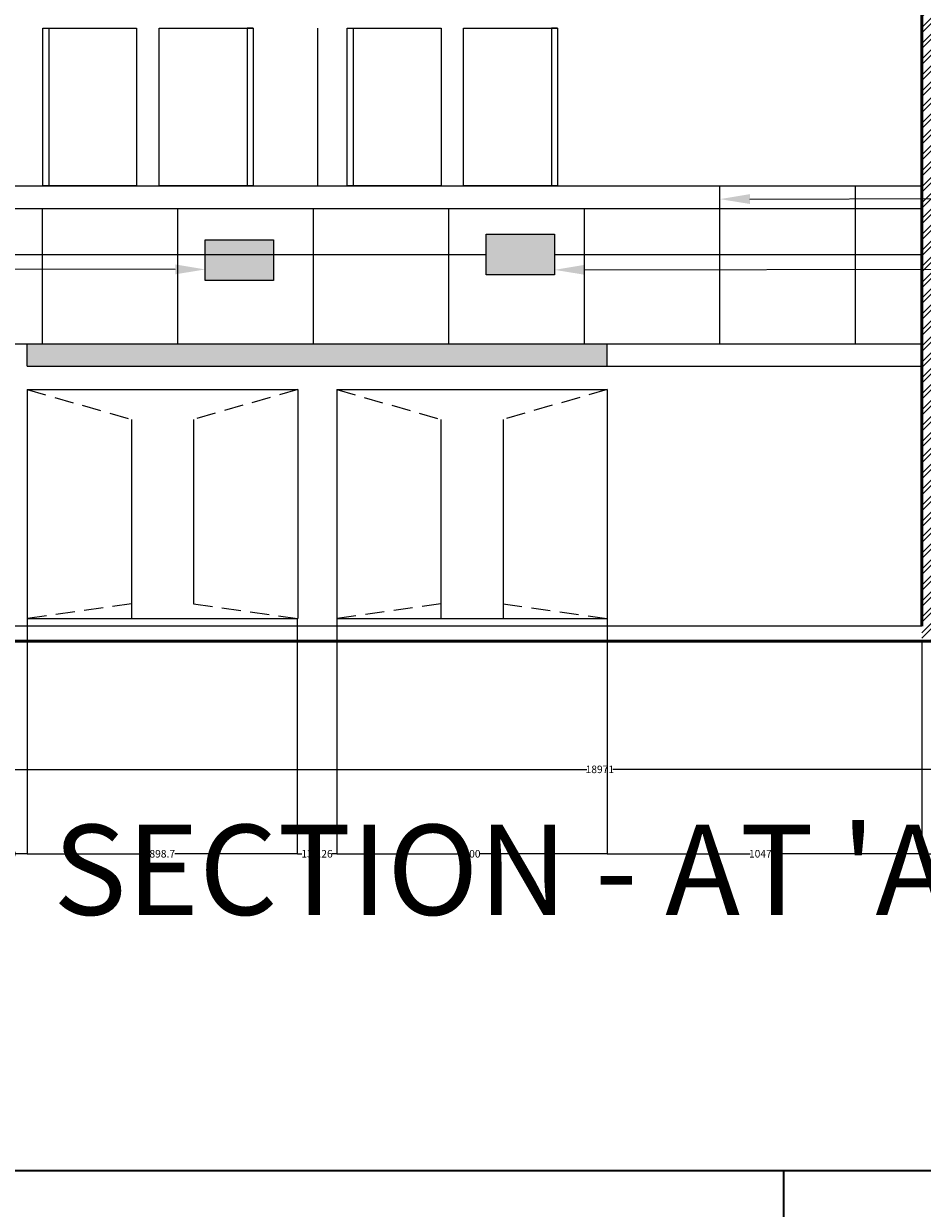
# Model space of a CAD drawing. Units: millimetres. Extents: x 1944 to 29915, y -10550 to 5909.
# Tile 15 of 24: x 13987 to 16977, y -1857 to 2086. Entities that reach past the tile are written whole.
import ezdxf
from ezdxf import colors
from ezdxf.entities.mleader import LeaderData, LeaderLine
from ezdxf.math import Vec2, Vec3

# ---------------------------------------------------------------- set-up
doc = ezdxf.new("R2010")
doc.units = ezdxf.units.MM
doc.header["$MEASUREMENT"] = 0
doc.linetypes.add('HIDDEN', pattern=[9.525, 6.35, -3.175])
for name, color, linetype, lineweight in [('A-ANNO-DIMS', 2, 'Continuous', 18), ('A-ANNO-TEXT', 7, 'Continuous', 25), ('A-ELEV', 3, 'Continuous', 18), ('A-ELEV-HIDN', 3, 'HIDDEN', 13), ('A-SECT', 7, 'Continuous', 35), ('A-WALL', 7, 'Continuous', 50), ('A-WALL-PATT', 8, 'Continuous', 18)]:
    doc.layers.add(name, color=color, linetype=linetype, lineweight=lineweight)
doc.styles.get("Standard").update_dxf_attribs({"font": 'arial.ttf'})
doc.dimstyles.get("Standard").update_dxf_attribs({"dimtxt": 25, "dimasz": 0.18, "dimexe": 0.18, "dimexo": 0.0625, "dimgap": 0.09, "dimtad": 0, "dimtih": 1, "dimtoh": 1, "dimdec": 0, "dimzin": 0, "dimdsep": 46, "dimtxsty": 'Standard', "dimcen": 0.09, "dimadec": 0, "dimazin": 0, "dimtfac": 1, "dimtdec": 0, "dimtofl": 0, "dimtmove": 0, "dimatfit": 3, "dimfxl": 1, "dimtolj": 1, "dimtzin": 0, "dimarcsym": 0})

# ---------------------------------------------------------------- blocks, each defined once
blk = doc.blocks.new('*D66')
at = {"layer": 'A-ANNO-DIMS', "color": 0, "lineweight": -2, "transparency": 16777216}
for p, q in [((13868.5, 105.8), (13868.5, -677)), ((13998.5, 105.8), (13998.5, -677)), ((13868.7, -676.8), (13907.1, -676.8)), ((13998.4, -676.8), (13960, -676.8))]:
    blk.add_line(p, q, dxfattribs=at)
at = {"layer": 'A-ANNO-DIMS', "color": 0, "transparency": 16777216}
for points in [[(13868.7, -676.8), (13868.7, -676.9), (13868.5, -676.8)], [(13998.4, -676.8), (13998.4, -676.9), (13998.5, -676.8)]]:
    blk.add_solid(points, dxfattribs=at)
at = {"layer": 'Defpoints', "color": 0, "transparency": 16777216}
for p in [(13868.5, 105.8), (13998.5, 105.8), (13998.5, -676.8)]:
    blk.add_point(p, dxfattribs=at)
at = {"layer": 'A-ANNO-DIMS', "color": 0, "transparency": 16777216, "insert": (13933.5, -676.8), "char_height": 25, "attachment_point": 5}
blk.add_mtext('\\A1;130', dxfattribs=at)
blk = doc.blocks.new('*D67')
at = {"layer": 'A-ANNO-DIMS', "color": 0, "lineweight": -2, "transparency": 16777216}
for p, q in [((13998.5, 105.8), (13998.5, -677)), ((14897.3, 105.8), (14897.3, -677)), ((13998.7, -676.8), (14405.6, -676.8)), ((14897.1, -676.8), (14490.2, -676.8))]:
    blk.add_line(p, q, dxfattribs=at)
at = {"layer": 'A-ANNO-DIMS', "color": 0, "transparency": 16777216}
for points in [[(13998.7, -676.8), (13998.7, -676.9), (13998.5, -676.8)], [(14897.1, -676.8), (14897.1, -676.9), (14897.3, -676.8)]]:
    blk.add_solid(points, dxfattribs=at)
at = {"layer": 'Defpoints', "color": 0, "transparency": 16777216}
for p in [(13998.5, 105.8), (14897.3, 105.8), (14897.3, -676.8)]:
    blk.add_point(p, dxfattribs=at)
at = {"layer": 'A-ANNO-DIMS', "color": 0, "transparency": 16777216, "insert": (14447.9, -676.8), "char_height": 25, "attachment_point": 5}
blk.add_mtext('\\A1;898.7', dxfattribs=at)
blk = doc.blocks.new('*D68')
at = {"layer": 'A-ANNO-DIMS', "color": 0, "lineweight": -2, "transparency": 16777216}
for p, q in [((14897.3, 105.8), (14897.3, -677)), ((15028.5, 105.8), (15028.5, -677)), ((14897.5, -676.8), (14912.1, -676.8)), ((15028.4, -676.8), (15013.7, -676.8))]:
    blk.add_line(p, q, dxfattribs=at)
at = {"layer": 'A-ANNO-DIMS', "color": 0, "transparency": 16777216}
for points in [[(14897.5, -676.8), (14897.5, -676.9), (14897.3, -676.8)], [(15028.4, -676.8), (15028.4, -676.9), (15028.5, -676.8)]]:
    blk.add_solid(points, dxfattribs=at)
at = {"layer": 'Defpoints', "color": 0, "transparency": 16777216}
for p in [(14897.3, 105.8), (15028.5, 105.8), (15028.5, -676.8)]:
    blk.add_point(p, dxfattribs=at)
at = {"layer": 'A-ANNO-DIMS', "color": 0, "transparency": 16777216, "insert": (14962.9, -676.8), "char_height": 25, "attachment_point": 5}
blk.add_mtext('\\A1;131.26', dxfattribs=at)
blk = doc.blocks.new('*D69')
at = {"layer": 'A-ANNO-DIMS', "color": 0, "lineweight": -2, "transparency": 16777216}
for p, q in [((15028.5, 105.8), (15028.5, -677)), ((15928.5, 105.8), (15928.5, -677)), ((15028.7, -676.8), (15450.9, -676.8)), ((15928.4, -676.8), (15506.2, -676.8))]:
    blk.add_line(p, q, dxfattribs=at)
at = {"layer": 'A-ANNO-DIMS', "color": 0, "transparency": 16777216}
for points in [[(15028.7, -676.8), (15028.7, -676.9), (15028.5, -676.8)], [(15928.4, -676.8), (15928.4, -676.9), (15928.5, -676.8)]]:
    blk.add_solid(points, dxfattribs=at)
at = {"layer": 'Defpoints', "color": 0, "transparency": 16777216}
for p in [(15028.5, 105.8), (15928.5, 105.8), (15928.5, -676.8)]:
    blk.add_point(p, dxfattribs=at)
at = {"layer": 'A-ANNO-DIMS', "color": 0, "transparency": 16777216, "insert": (15478.5, -676.8), "char_height": 25, "attachment_point": 5}
blk.add_mtext('\\A1;900', dxfattribs=at)
blk = doc.blocks.new('*D70')
at = {"layer": 'A-ANNO-DIMS', "color": 0, "lineweight": -2, "transparency": 16777216}
for p, q in [((15928.548289, 105.774608), (15928.548289, -677.022892)), ((16975.669859, 30.774608), (16975.669859, -677.022892)), ((15928.728289, -676.842892), (16403.715868, -676.842892)), ((16975.489859, -676.842892), (16500.50228, -676.842892))]:
    blk.add_line(p, q, dxfattribs=at)
at = {"layer": 'A-ANNO-DIMS', "color": 0, "transparency": 16777216}
for points in [[(15928.728289, -676.812892), (15928.728289, -676.872892), (15928.548289, -676.842892)], [(16975.489859, -676.812892), (16975.489859, -676.872892), (16975.669859, -676.842892)]]:
    blk.add_solid(points, dxfattribs=at)
at = {"layer": 'Defpoints', "color": 0, "transparency": 16777216}
for p in [(15928.548289, 105.837108), (16975.669859, 30.837108), (16975.669859, -676.842892)]:
    blk.add_point(p, dxfattribs=at)
at = {"layer": 'A-ANNO-DIMS', "color": 0, "transparency": 16777216, "insert": (16452.109074, -676.842892), "char_height": 25, "attachment_point": 5}
blk.add_mtext('\\A1;1047.1', dxfattribs=at)
blk = doc.blocks.new('*D71')
at = {"layer": 'A-ANNO-DIMS', "color": 0, "lineweight": -2, "transparency": 16777216}
for p, q in [((16975.7, 30.8), (16975.7, -677)), ((17205.7, 30.8), (17205.7, -677)), ((16975.8, -676.8), (17062.8, -676.8)), ((17205.5, -676.8), (17118.5, -676.8))]:
    blk.add_line(p, q, dxfattribs=at)
at = {"layer": 'A-ANNO-DIMS', "color": 0, "transparency": 16777216}
for points in [[(16975.8, -676.8), (16975.8, -676.9), (16975.7, -676.8)], [(17205.5, -676.8), (17205.5, -676.9), (17205.7, -676.8)]]:
    blk.add_solid(points, dxfattribs=at)
at = {"layer": 'Defpoints', "color": 0, "transparency": 16777216}
for p in [(16975.7, 30.8), (17205.7, 30.8), (17205.7, -676.8)]:
    blk.add_point(p, dxfattribs=at)
at = {"layer": 'A-ANNO-DIMS', "color": 0, "transparency": 16777216, "insert": (17090.7, -676.8), "char_height": 25, "attachment_point": 5}
blk.add_mtext('\\A1;230', dxfattribs=at)
blk = doc.blocks.new('*D85')
at = {"layer": 'A-ANNO-DIMS', "color": 0, "lineweight": -2, "transparency": 16777216}
for p, q in [((6418.3, -1730.7), (6418.3, -395.6)), ((6418.5, -395.8), (15860.3, -395.8)), ((25389.1, -395.8), (15947.3, -395.8)), ((25389.3, -1846.5), (25389.3, -395.6))]:
    blk.add_line(p, q, dxfattribs=at)
at = {"layer": 'A-ANNO-DIMS', "color": 0, "transparency": 16777216}
for points in [[(6418.5, -395.7), (6418.5, -395.8), (6418.3, -395.8)], [(25389.1, -395.7), (25389.1, -395.8), (25389.3, -395.8)]]:
    blk.add_solid(points, dxfattribs=at)
at = {"layer": 'Defpoints', "color": 0, "transparency": 16777216}
for p in [(25389.3, -395.8), (6418.3, -1730.8), (25389.3, -1846.5)]:
    blk.add_point(p, dxfattribs=at)
at = {"layer": 'A-ANNO-DIMS', "color": 0, "transparency": 16777216, "insert": (15903.8, -395.8), "char_height": 25, "attachment_point": 5}
blk.add_mtext('\\A1;18971', dxfattribs=at)

msp = doc.modelspace()

# ---------------------------------------------------------------- hatches: boundary and pattern name
at = {"layer": 'A-ELEV'}
h = msp.add_hatch(color=256, dxfattribs=at)
h.dxf.hatch_style = 1
h.paths.add_polyline_path([(15525.455, 1385.243), (15525.455, 1249.658), (15752.828, 1249.658), (15752.828, 1385.243)])
h = msp.add_hatch(color=256, dxfattribs=at)
h.dxf.hatch_style = 1
h.paths.add_polyline_path([(14591.122, 1366.385), (14591.122, 1230.801), (14818.496, 1230.801), (14818.496, 1366.385)])
h = msp.add_hatch(color=256, dxfattribs=at)
h.dxf.hatch_style = 1
h.paths.add_polyline_path([(15928.548, 945.657), (15928.548, 1020.657), (13998.548, 1020.657), (13998.548, 945.657)])
at = {"layer": 'A-WALL-PATT'}
h = msp.add_hatch(dxfattribs=at)
h.set_pattern_fill('ANSI32', color=256, scale=100)
h.paths.add_polyline_path([(17205.67, 2905.657), (16975.67, 2905.657), (16975.67, 30.837), (17205.67, 30.837)])

# ---------------------------------------------------------------- linework, layer by layer
at = {"layer": 'A-ELEV'}
for p, q in [((14050.393, 2070.657), (14070.393, 2070.657)), ((14070.393, 2070.657), (14070.393, 1545.657)), ((14750.084, 2070.657), (14730.084, 2070.657)), ((14730.084, 2070.657), (14730.084, 1545.657)), ((14964.935, 2070.657), (14964.935, 1545.657)), ((15063.189, 2070.657), (15083.189, 2070.657)), ((15083.189, 2070.657), (15083.189, 1545.657)), ((15762.881, 2070.657), (15742.881, 2070.657)), ((15742.881, 2070.657), (15742.881, 1545.657)), ((12891.548, 1545.657), (16975.67, 1545.657)), ((16303.171, 1020.657), (16303.171, 1545.657)), ((16753.882, 1545.657), (16753.882, 1020.657)), ((12891.548, 1470.657), (16975.67, 1470.657)), ((14049.617, 1020.657), (14049.617, 1470.657)), ((14500.328, 1020.657), (14500.328, 1470.657)), ((14951.039, 1020.657), (14951.039, 1470.657)), ((15401.75, 1020.657), (15401.75, 1470.657)), ((15852.46, 1020.657), (15852.46, 1470.657)), ((12891.548, 1317.451), (15525.455, 1317.451)), ((15752.828, 1317.451), (16975.67, 1317.451)), ((12891.548, 1020.657), (16975.67, 1020.657)), ((13998.548, 945.657), (13998.548, 1020.657)), ((15928.548, 945.657), (15928.548, 1020.657)), ((13998.548, 945.657), (16975.67, 945.657)), ((13998.548, 868.657), (14898.548, 868.657)), ((13998.548, 868.657), (13998.548, 105.837)), ((14898.548, 868.657), (14898.548, 105.657)), ((15028.548, 868.657), (15028.548, 105.657)), ((15028.548, 868.657), (15928.548, 868.657)), ((15928.548, 868.657), (15928.548, 105.837)), ((14345.349, 768.181), (14345.349, 105.837)), ((14551.747, 768.181), (14551.747, 155.141)), ((15375.349, 768.181), (15375.349, 105.837)), ((15581.747, 768.181), (15581.747, 105.837)), ((16975.67, 81.017), (12891.548, 81.017)), ((13998.548, 105.837), (14345.349, 105.837)), ((14345.349, 105.837), (14897.287, 105.837)), ((14897.287, 105.837), (14898.548, 105.837)), ((15028.548, 105.837), (15375.349, 105.837)), ((15375.349, 105.837), (15581.747, 105.837)), ((15581.747, 105.837), (15928.548, 105.837)), ((12891.548, 30.837), (16975.67, 30.837)), ((13998.548, 30.837), (13998.548, 30.657)), ((13998.548, 30.657), (14898.548, 30.657)), ((14898.548, 30.837), (14898.548, 30.657)), ((15028.548, 30.837), (15028.548, 30.657)), ((15028.548, 30.657), (15928.548, 30.657))]:
    msp.add_line(p, q, dxfattribs=at)
for points in [[(14050.393, 2070.657), (14362.739, 2070.657), (14362.739, 1545.657), (14050.393, 1545.657)], [(14437.739, 2070.657), (14750.084, 2070.657), (14750.084, 1545.657), (14437.739, 1545.657)], [(15063.189, 2070.657), (15375.535, 2070.657), (15375.535, 1545.657), (15063.189, 1545.657)], [(15450.535, 2070.657), (15762.881, 2070.657), (15762.881, 1545.657), (15450.535, 1545.657)], [(15525.455, 1385.243), (15752.828, 1385.243), (15752.828, 1249.658), (15525.455, 1249.658)], [(14591.122, 1366.385), (14818.496, 1366.385), (14818.496, 1230.801), (14591.122, 1230.801)]]:
    msp.add_lwpolyline(points, close=True, dxfattribs=at)
at = {"layer": 'A-ELEV-HIDN', "ltscale": 10}
for p, q in [((13998.548, 868.657), (14345.349, 768.181)), ((14898.548, 868.657), (14551.747, 768.181)), ((15028.548, 868.657), (15375.349, 768.181)), ((15928.548, 868.657), (15581.747, 768.181)), ((14345.349, 155.321), (13998.548, 105.837)), ((14551.747, 155.141), (14898.548, 105.657)), ((15375.349, 155.141), (15028.548, 105.657)), ((15581.747, 155.141), (15928.548, 105.657))]:
    msp.add_line(p, q, dxfattribs=at)
at = {"layer": 'A-SECT'}
for p, q in [((6418.315, -1730.752), (16516.552, -1730.752)), ((16516.552, -2630.752), (16516.552, -1730.752)), ((16516.552, -1730.752), (20985.45, -1730.752))]:
    msp.add_line(p, q, dxfattribs=at)
at = {"layer": 'A-WALL'}
for p, q in [((16975.67, 81.017), (16975.67, 3230.657)), ((24504.139, 30.837), (12776.548, 30.837))]:
    msp.add_line(p, q, dxfattribs=at)

# ---------------------------------------------------------------- texts
at = {"layer": 'A-ANNO-TEXT'}
msp.add_text("SECTION - AT 'A'", height=300, dxfattribs=at).set_placement((14085.235, -880.236))

# ---------------------------------------------------------------- dimensions: what is measured, and where the dimension line sits
at = {"layer": 'A-ANNO-DIMS'}
for base, p1, p2, override, picture, middle in [((13998.548, -676.843), (13868.548, 105.837), (13998.548, 105.837), {"dimdec": 0, "dimlfac": 1, "dimrnd": 0, "dimzin": 0, "dimdsep": 46, "dimlunit": 2}, '*D66', (13933.548, -676.843)), ((14897.287, -676.843), (13998.548, 105.837), (14897.287, 105.837), {"dimdec": 1, "dimlfac": 1, "dimrnd": 0, "dimzin": 0, "dimdsep": 46, "dimlunit": 2}, '*D67', (14447.918, -676.843)), ((15028.548, -676.843), (14897.287, 105.837), (15028.548, 105.837), {"dimdec": 2, "dimlfac": 1, "dimrnd": 0, "dimzin": 0, "dimdsep": 46, "dimlunit": 2}, '*D68', (14962.918, -676.843)), ((15928.548, -676.843), (15028.548, 105.837), (15928.548, 105.837), {"dimdec": 0, "dimlfac": 1, "dimrnd": 0, "dimzin": 0, "dimdsep": 46, "dimlunit": 2}, '*D69', (15478.548, -676.843)), ((16975.67, -676.843), (15928.548, 105.837), (16975.67, 30.837), {"dimdec": 1, "dimlfac": 1, "dimrnd": 0, "dimzin": 0, "dimdsep": 46, "dimlunit": 2}, '*D70', (16452.109, -676.843)), ((17205.67, -676.843), (16975.67, 30.837), (17205.67, 30.837), {"dimdec": 0, "dimlfac": 1, "dimrnd": 0, "dimzin": 0, "dimdsep": 46, "dimlunit": 2}, '*D71', (17090.67, -676.843)), ((25389.297, -395.752), (6418.315, -1730.752), (25389.297, -1846.542), {"dimdec": 0, "dimlfac": 1, "dimrnd": 0, "dimzin": 0, "dimdsep": 46, "dimlunit": 2}, '*D85', (15903.806, -395.752))]:
    dim = msp.add_linear_dim(base=base, p1=p1, p2=p2, dimstyle='Standard', override=override, dxfattribs=at)
    dim.commit()
    dim.dimension.update_dxf_attribs({"geometry": picture, "text_midpoint": middle})

# ---------------------------------------------------------------- leaders
at = {"layer": 'A-ANNO-TEXT'}
ml = msp.add_multileader_mtext('Standard', dxfattribs=at)
ml.set_content('TILE ', color=256)
ml.set_leader_properties()
ml.build(insert=Vec2(0, 0))
ml.multileader.update_dxf_attribs({"dogleg_length": 0.36, "arrow_head_size": 100})
ctx = ml.context
ctx.base_point, ctx.char_height, ctx.arrow_head_size, ctx.landing_gap_size, ctx.plane_origin = Vec3(17906.299, 1505.142), 100, 100, 0.09, Vec3(17905.939, 1505.142)
notes = []
notes.append((ctx, [(0, (1, 1, 0), (17905.939, 1505.142), (1, 0), 0.36, [(0, [(16303.171, 1501.973)], 0, [])])]))
ctx.mtext.insert, ctx.mtext.flow_direction = Vec3(17906.389, 1555.142), 5
ml = msp.add_multileader_mtext('Standard', dxfattribs=at)
ml.set_content('15 AMP POWER POINT \\PFOR GEYSER ', color=256)
ml.set_leader_properties()
ml.build(insert=Vec2(0, 0))
ml.multileader.update_dxf_attribs({"dogleg_length": 0.36, "arrow_head_size": 100})
ctx = ml.context
ctx.base_point, ctx.char_height, ctx.arrow_head_size, ctx.landing_gap_size, ctx.plane_origin = Vec3(10908.052, 1271.067), 100, 100, 0.09, Vec3(12988.354, 1271.067)
ctx.text_align_type = 2
notes.append((ctx, [(0, (1, 1, 0), (12988.354, 1271.067), (-1, 0), 568.936, [(0, [(14591.122, 1267.898)], 0, [])])]))
ctx.mtext.insert, ctx.mtext.alignment, ctx.mtext.flow_direction = Vec3(12419.329, 1321.919), 3, 5
ml = msp.add_multileader_mtext('Standard', dxfattribs=at)
ml.set_content('15 AMP\\PPOWER POINT \\PFOR MIXER ', color=256)
ml.set_leader_properties()
ml.build(insert=Vec2(0, 0))
ml.multileader.update_dxf_attribs({"dogleg_length": 0.36, "arrow_head_size": 100})
ctx = ml.context
ctx.base_point, ctx.char_height, ctx.arrow_head_size, ctx.landing_gap_size, ctx.plane_origin = Vec3(17355.956, 1269.694), 100, 100, 0.09, Vec3(17355.596, 1269.694)
notes.append((ctx, [(0, (1, 1, 0), (17355.596, 1269.694), (1, 0), 0.36, [(0, [(15752.828, 1266.525)], 0, [])])]))
ctx.mtext.insert, ctx.mtext.flow_direction = Vec3(17356.046, 1320.547), 5
for ctx, leaders in notes:
    for number, flags, end, landing, length, lines in leaders:
        leader = LeaderData()
        leader.index, (leader.has_last_leader_line, leader.has_dogleg_vector, leader.attachment_direction) = number, flags
        leader.last_leader_point, leader.dogleg_vector, leader.dogleg_length = Vec3(end), Vec3(landing), length
        for number, points, colour, breaks in lines:
            line = LeaderLine()
            line.index, line.vertices, line.color, line.breaks = number, Vec3.list(points), colors.encode_raw_color(colour), breaks
            leader.lines.append(line)
        ctx.leaders.append(leader)

doc.saveas('drawing.dxf')
